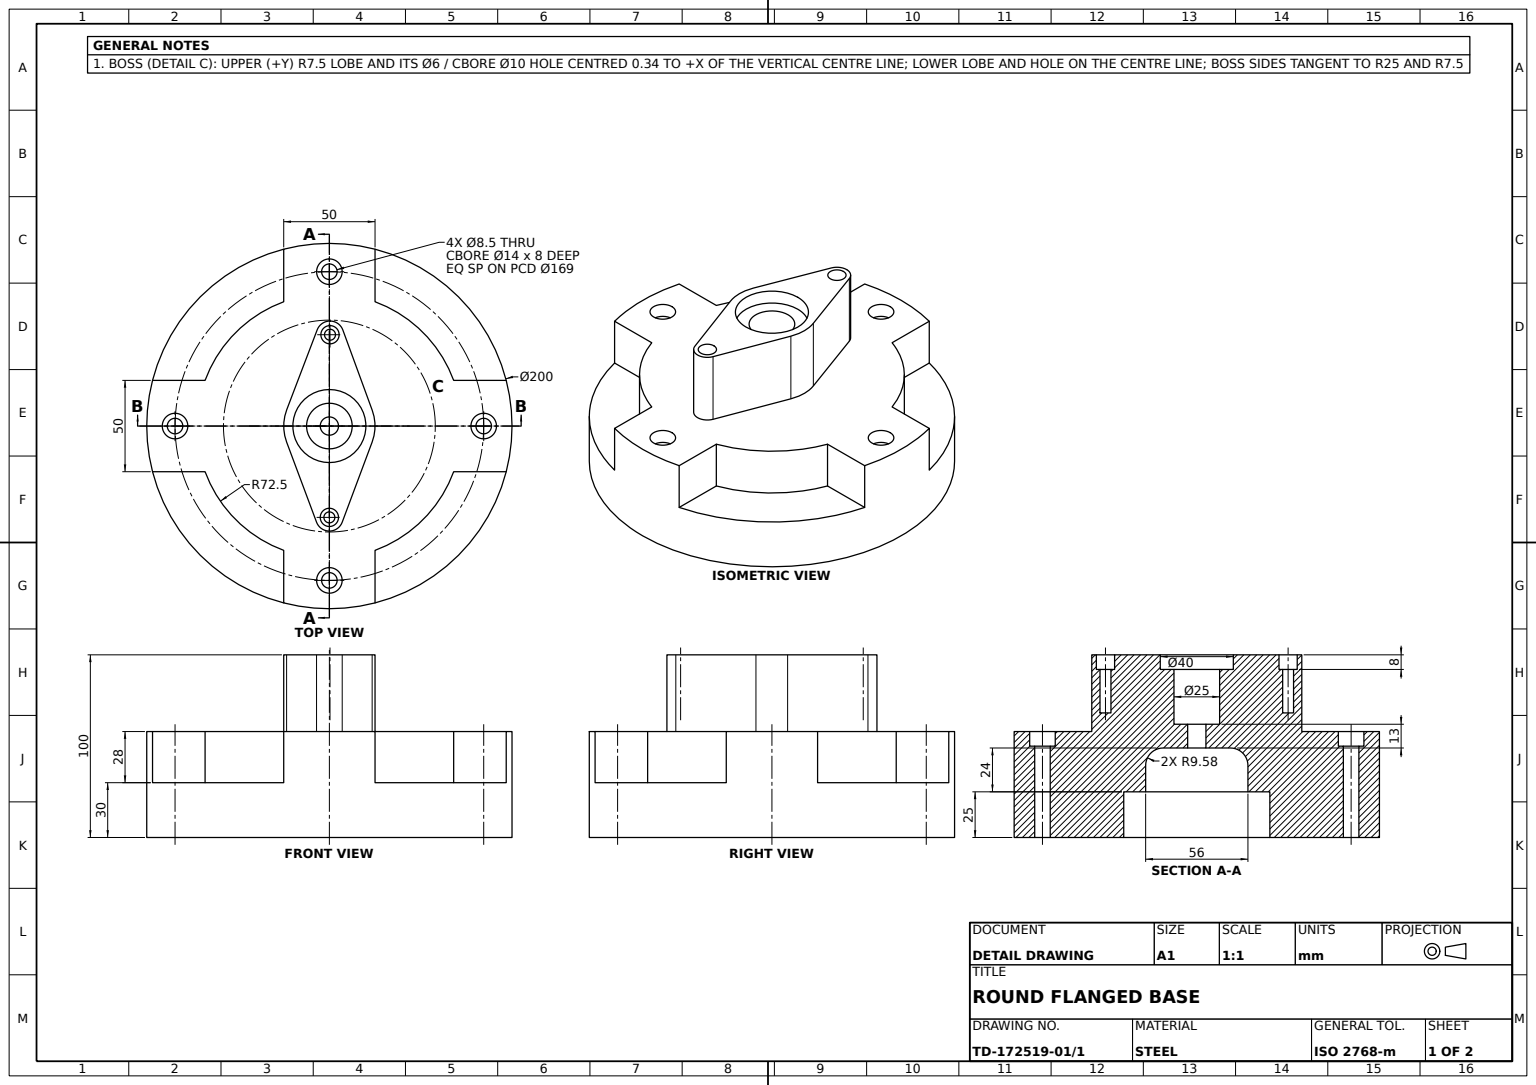
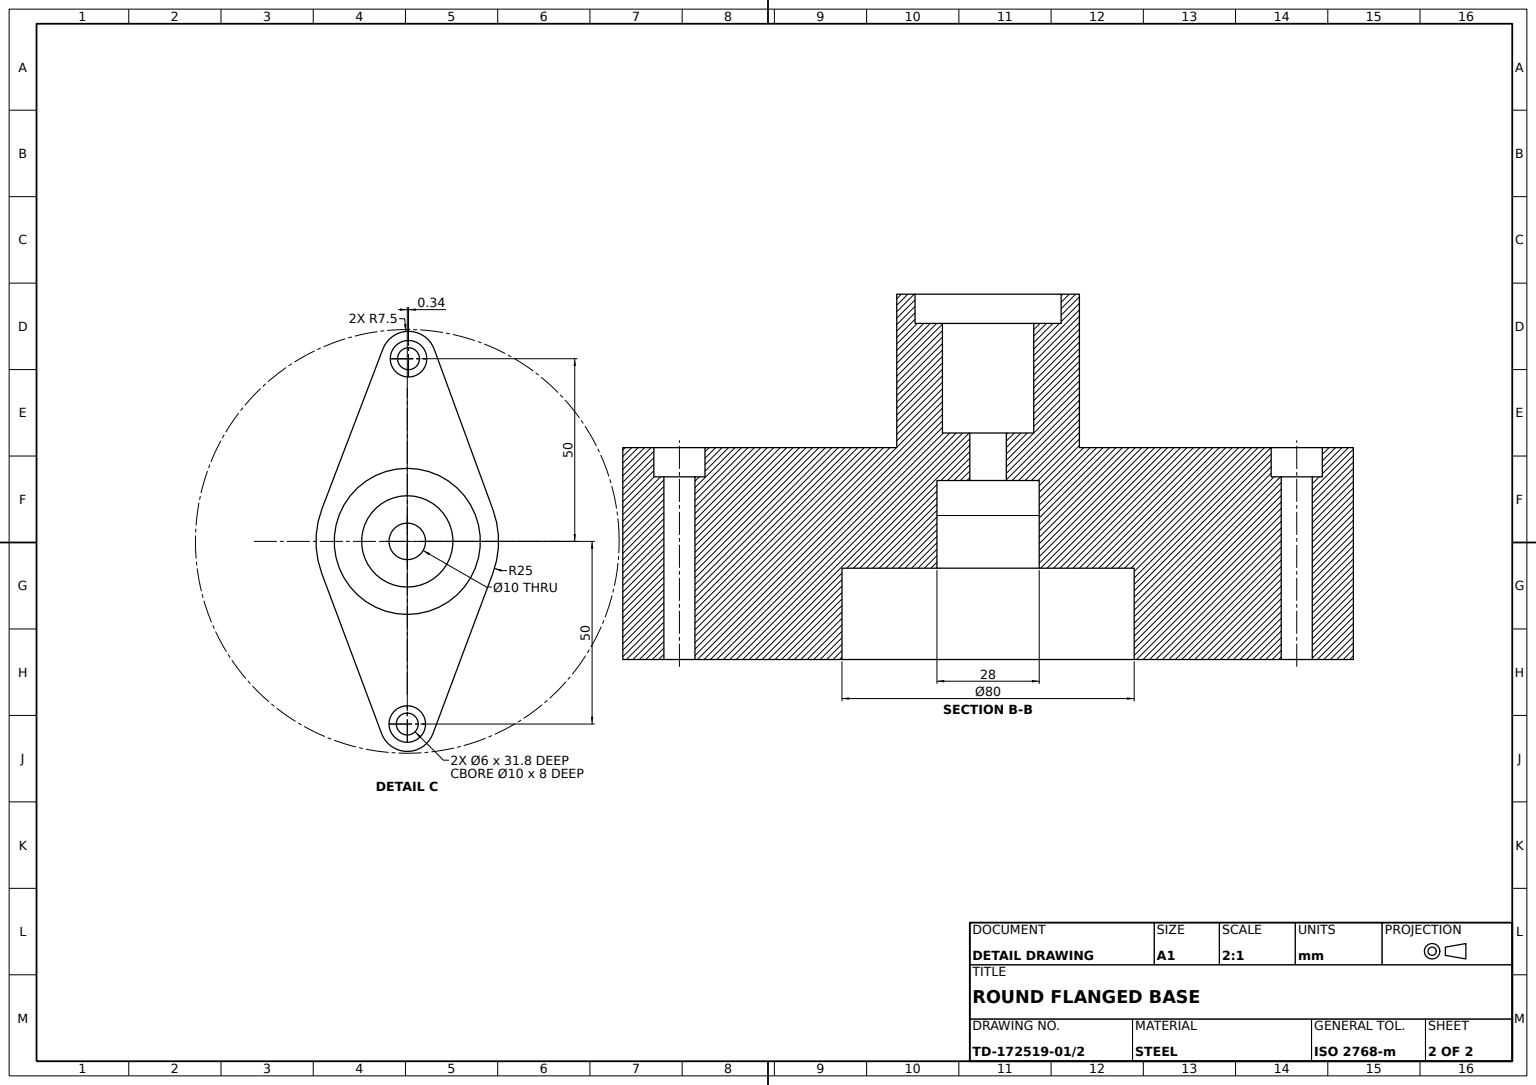
SolidWorks part; units mm, degrees
material "Plain Carbon Steel"
ref_plane "Front Plane" through (0, 0, 0) normal (0, 0, 1) x (1, 0, 0)
ref_plane "Top Plane" through (0, 0, 0) normal (0, 1, 0) x (1, 0, 0)
ref_plane "Right Plane" through (0, 0, 0) normal (1, 0, 0) x (0, 0, -1)
sketch "Base Flange Sketch" plane through (0, 0, 0) normal (0, 1, 0) x (1, 0, 0)
  circle A0 centre (0, 0) radius 100
  dimension "D1" = 200
extrude "Base Flange Ø200" add sketch "Base Flange Sketch" along normal blind 30
sketch "Mounting Pad Sketch" plane through (0, 30, 0) normal (0, 1, 0) x (1, 0, 0)
  line L0 (68.0533, 25) -> (96.8246, 25)
  line L2 (-25, 68.0533) -> (-25, 96.8246)
  line L4 (25, 68.0533) -> (25, 96.8246)
  line L5 (68.0533, -25) -> (96.8246, -25)
  line L6 (25, -68.0533) -> (25, -96.8246)
  line L7 (-25, -68.0533) -> (-25, -96.8246)
  line L8 (-68.0533, -25) -> (-96.8246, -25)
  line L9 (-68.0533, 25) -> (-96.8246, 25)
  arc A0 (-25, 68.0533) -> (-68.0533, 25) centre (0, 0) ccw
  arc A1 (25, 96.8246) -> (-25, 96.8246) centre (0, 0) ccw
  arc A2 (96.8246, -25) -> (96.8246, 25) centre (0, 0) ccw
  arc A3 (-25, -96.8246) -> (25, -96.8246) centre (0, 0) ccw
  arc A4 (-96.8246, 25) -> (-96.8246, -25) centre (0, 0) ccw
  arc A5 (-68.0533, -25) -> (-25, -68.0533) centre (0, 0) ccw
  arc A6 (25, -68.0533) -> (68.0533, -25) centre (0, 0) ccw
  arc A7 (68.0533, 25) -> (25, 68.0533) centre (0, 0) ccw
  point P3 (0, 72.5)
  dimension "D1" = 145
  dimension "D3" = 68.0533
  dimension "D2" = 4
  dimension "D4" = 96.8246
  dimension "D5" = 68.0533
extrude "Mounting Pad" add sketch "Mounting Pad Sketch" along normal blind 28
sketch "Mounting Counterbores Sketch" plane through (0, 58, 0) normal (0, 1, 0) x (1, 0, 0)
  circle A1 centre (0, 84.5) radius 7
  circle A2 centre (84.5, 0) radius 7
  circle A3 centre (0, -84.5) radius 7
  circle A4 centre (-84.5, 0) radius 7
  dimension "D1" = 84.5
  dimension "D2" = 14
  dimension "D4" = 84.5
  dimension "D5" = 84.5
  dimension "D6" = 84.5
  dimension "D3" = 4
extrude "Mounting Counterbores 4xØ14" cut sketch "Mounting Counterbores Sketch" against normal blind 8
sketch "Mounting Holes Sketch" plane through (0, 50, 0) normal (0, 1, 0) x (1, 0, 0)
  circle A0 centre (0, 84.5) radius 4.25
  circle A1 centre (84.5, 0) radius 4.25
  circle A2 centre (0, -84.5) radius 4.25
  circle A3 centre (-84.5, 0) radius 4.25
  dimension "D1" = 8.5
  dimension "D3" = 84.5
  dimension "D4" = 84.5
  dimension "D2" = 4
extrude "Mounting Holes 4xØ8.5" cut sketch "Mounting Holes Sketch" against normal blind 50
sketch "Support Boss Sketch" plane through (0, 58, 0) normal (0, 1, 0) x (1, 0, 0)
  line L0 (-6.6704, 52.6712) -> (-23.3592, 8.9078)
  line L1 (7.3805, 52.5764) -> (23.4772, 8.5918)
  line L2 (-7.0256, -52.625) -> (-23.4187, -8.75)
  line L3 (7.0256, -52.625) -> (23.4187, -8.75)
  arc A0 (23.4187, -8.75) -> (23.4772, 8.5918) centre (0, 0) ccw
  arc A1 (7.3805, 52.5764) -> (-6.6704, 52.6712) centre (0.3373, 49.9989) ccw
  arc A2 (-7.0256, -52.625) -> (7.0256, -52.625) centre (0, -50) ccw
  arc A3 (-23.3592, 8.9078) -> (-23.4187, -8.75) centre (0, 0) ccw
  dimension "D1" = 50
  dimension "D2" = 15
  dimension "D3" = 15
  dimension "D4" = 50
  dimension "D5" = 50
  dimension "D6" = 41.0911
  dimension "D7" = 23.4187
extrude "Support Boss" add sketch "Support Boss Sketch" along normal blind 42
sketch "Bearing Counterbore Sketch" plane through (0, 100, 0) normal (0, 1, 0) x (1, 0, 0)
  circle A0 centre (0, 0) radius 20
  dimension "D1" = 40
extrude "Bearing Counterbore Ø40" cut sketch "Bearing Counterbore Sketch" against normal blind 8
sketch "Bearing Bore Sketch" plane through (0, 92, 0) normal (0, 1, 0) x (1, 0, 0)
  circle A0 centre (0, 0) radius 12.5
  dimension "D1" = 25
extrude "Bearing Bore Ø25" cut sketch "Bearing Bore Sketch" against normal blind 30
sketch "Through Bore Sketch" plane through (0, 62, 0) normal (0, 1, 0) x (1, 0, 0)
  circle A0 centre (0, 0) radius 5
  dimension "D1" = 10
extrude "Through Bore Ø10" cut sketch "Through Bore Sketch" against normal blind 13
sketch "Underside Recess Sketch" plane through (0, 0, 0) normal (0, -1, 0) x (1, 0, 0)
  circle A0 centre (0, 0) radius 40
  dimension "D1" = 80
extrude "Underside Recess Ø80" cut sketch "Underside Recess Sketch" against normal blind 25
ref_plane "Plane2" through (0, 0, 0) normal (1, 0, 0) x (0, 0, -1)
sketch "Side Slot Sketch" plane through (0, 0, 0) normal (1, 0, 0) x (0, 0, -1)
  line L0 (-40, 25) -> (40, 25) construction
  line L1 (-28, 25) -> (28, 25)
  line L2 (-28, 25) -> (-28, 39.42)
  line L3 (-18.42, 49) -> (18.42, 49)
  line L4 (28, 25) -> (28, 39.42)
  arc A0 (28, 39.42) -> (18.42, 49) centre (18.42, 39.42) ccw
  arc A1 (-18.42, 49) -> (-28, 39.42) centre (-18.42, 39.42) ccw
  point P9 (28, 49)
  dimension "D4" = 9.58
  dimension "D1" = 28
  dimension "D2" = 56
  dimension "D3" = 24
extrude "Side Slot" cut sketch "Side Slot Sketch" against normal mid plane 28
sketch "Boss Hole Counterbores Sketch" plane through (0, 100, 0) normal (0, 1, 0) x (1, 0, 0)
  circle A0 centre (0.3373, 49.9989) radius 5
  circle A1 centre (0, -50) radius 5
  dimension "D1" = 10
  dimension "D2" = 10
extrude "Boss Hole Counterbores 2xØ10" cut sketch "Boss Hole Counterbores Sketch" against normal blind 8
sketch "Boss Pin Holes Sketch" plane through (0, 92, 0) normal (0, 1, 0) x (1, 0, 0)
  circle A0 centre (0.3373, 49.9989) radius 3
  circle A1 centre (0, -50) radius 3
  dimension "D1" = 6
  dimension "D2" = 6
extrude "Boss Pin Holes 2xØ6" cut sketch "Boss Pin Holes Sketch" against normal blind 23.8
